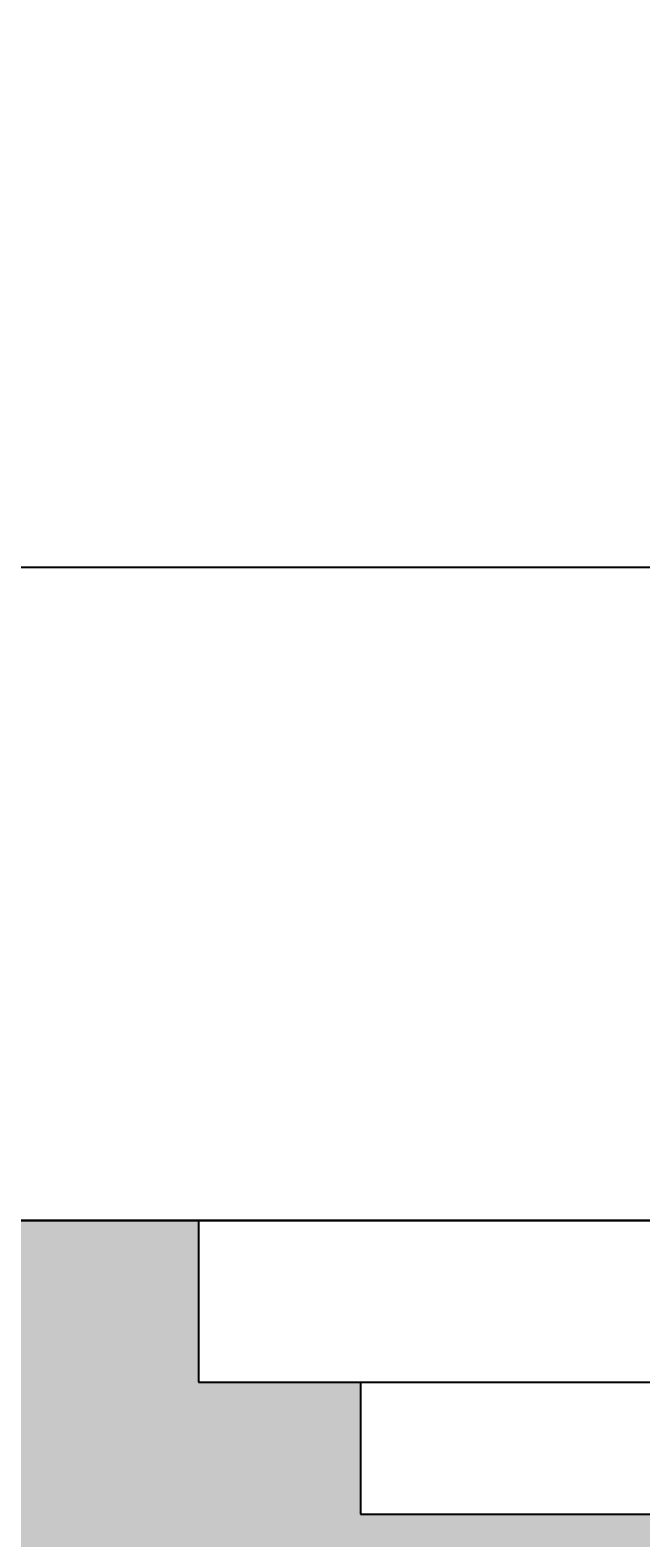
# Model space of a CAD drawing. Units: inches. Extents: x 2549 to 3108, y 1683 to 2362.
# Tile 5 of 30: x 2970 to 3018, y 1861 to 1979. Entities that reach past the tile are written whole.
import ezdxf

# ---------------------------------------------------------------- set-up
doc = ezdxf.new("R2010")
doc.units = ezdxf.units.IN
for name, color, linetype, lineweight in [('A-ANNO-DIMS', 2, 'Continuous', 18), ('A-FLOR', 7, 'Continuous', 25), ('A-FLOR-STRS', 7, 'Continuous', 25)]:
    doc.layers.add(name, color=color, linetype=linetype, lineweight=lineweight)
doc.layers.add('C-PKNG-VEHI-PATT', color=251, linetype='Continuous', lineweight=13, true_color=0x636466)
doc.layers.add('C-PVMT-PATT', color=9, linetype='Continuous', lineweight=13, true_color=0xc7c8ca)
doc.styles.get("Standard").update_dxf_attribs({"font": 'arial.ttf'})
doc.dimstyles.get("Standard").update_dxf_attribs({"dimtxt": 0.18, "dimasz": 0.18, "dimexe": 0.18, "dimexo": 0.0625, "dimgap": 0.09, "dimtad": 0, "dimtih": 1, "dimtoh": 1, "dimdec": 4, "dimzin": 0, "dimdsep": 46, "dimtxsty": 'Standard', "dimcen": 0.09, "dimadec": 0, "dimazin": 0, "dimtfac": 1, "dimtdec": 4, "dimtofl": 0, "dimtmove": 0, "dimatfit": 3, "dimfxl": 1, "dimtolj": 1, "dimtzin": 0, "dimarcsym": 0})

# ---------------------------------------------------------------- blocks, each defined once
blk = doc.blocks.new('*D46')
at = {"layer": 'A-ANNO-DIMS', "color": 0, "lineweight": -2, "transparency": 16777216}
for p, q in [((2812.642666, 2140.461244), (2812.642666, 1683.443744)), ((3034.642666, 2134.461244), (3034.642666, 1683.443744)), ((2812.822666, 1683.623744), (2923.35320488131, 1683.623744)), ((3034.462666, 1683.623744), (2923.932127118691, 1683.623744))]:
    blk.add_line(p, q, dxfattribs=at)
at = {"layer": 'A-ANNO-DIMS', "color": 0, "transparency": 16777216}
for points in [[(2812.822666, 1683.653744), (2812.822666, 1683.593744), (2812.642666, 1683.623744)], [(3034.462666, 1683.653744), (3034.462666, 1683.593744), (3034.642666, 1683.623744)]]:
    blk.add_solid(points, dxfattribs=at)
at = {"layer": 'Defpoints', "color": 0, "transparency": 16777216}
for p in [(2812.642666, 2140.523744), (3034.642666, 2134.523744), (3034.642666, 1683.623744)]:
    blk.add_point(p, dxfattribs=at)
at = {"layer": 'A-ANNO-DIMS', "color": 0, "transparency": 16777216, "insert": (2923.642666000001, 1683.623744), "char_height": 0.18, "attachment_point": 5}
blk.add_mtext('\\A1;222', dxfattribs=at)
blk = doc.blocks.new('*D56')
at = {"layer": 'A-ANNO-DIMS', "color": 0, "lineweight": -2, "transparency": 16777216}
for p, q in [((3043.580166000001, 1936.523744000001), (2549.424763000002, 1936.523744000001)), ((2549.604763000002, 1936.343744000001), (2549.604763000002, 1911.205647137791)), ((2549.604763000002, 1885.703744000001), (2549.604763000002, 1910.841840862211)), ((3043.580166000001, 1885.523744000001), (2549.424763000002, 1885.523744000001))]:
    blk.add_line(p, q, dxfattribs=at)
at = {"layer": 'A-ANNO-DIMS', "color": 0, "transparency": 16777216}
for points in [[(2549.574763000002, 1936.343744000001), (2549.634763000002, 1936.343744000001), (2549.604763000002, 1936.523744000001)], [(2549.574763000002, 1885.703744000001), (2549.634763000002, 1885.703744000001), (2549.604763000002, 1885.523744000001)]]:
    blk.add_solid(points, dxfattribs=at)
at = {"layer": 'Defpoints', "color": 0, "transparency": 16777216}
for p in [(2549.604763000002, 1936.523744000001), (3043.642666000001, 1936.523744000001), (3043.642666000001, 1885.523744000001)]:
    blk.add_point(p, dxfattribs=at)
at = {"layer": 'A-ANNO-DIMS', "color": 0, "transparency": 16777216, "insert": (2549.604763000002, 1911.023743999999), "char_height": 0.18, "attachment_point": 5}
blk.add_mtext('\\A1;51', dxfattribs=at)
blk = doc.blocks.new('*D57')
at = {"layer": 'A-ANNO-DIMS', "color": 0, "lineweight": -2, "transparency": 16777216}
for p, q in [((2965.93514, 1936.586244), (2965.93514, 2362.322518)), ((2966.11514, 2362.142518), (2999.912081717599, 2362.142518)), ((3034.462666, 2362.142518), (3000.665724282401, 2362.142518)), ((3034.642666, 1936.586244), (3034.642666, 2362.322518))]:
    blk.add_line(p, q, dxfattribs=at)
at = {"layer": 'A-ANNO-DIMS', "color": 0, "transparency": 16777216}
for points in [[(2966.11514, 2362.172518), (2966.11514, 2362.112518), (2965.93514, 2362.142518)], [(3034.462666, 2362.172518), (3034.462666, 2362.112518), (3034.642666, 2362.142518)]]:
    blk.add_solid(points, dxfattribs=at)
at = {"layer": 'Defpoints', "color": 0, "transparency": 16777216}
for p in [(3034.642666, 2362.142518), (2965.93514, 1936.523744), (3034.642666, 1936.523744)]:
    blk.add_point(p, dxfattribs=at)
at = {"layer": 'A-ANNO-DIMS', "color": 0, "transparency": 16777216, "insert": (3000.288903, 2362.142518), "char_height": 0.18, "attachment_point": 5}
blk.add_mtext('\\A1;68.71', dxfattribs=at)

msp = doc.modelspace()

# ---------------------------------------------------------------- hatches: boundary and pattern name
at = {"layer": 'C-PKNG-VEHI-PATT'}
h = msp.add_hatch(color=256, dxfattribs=at)
h.dxf.hatch_style = 1
edge = h.paths.add_edge_path()
edge.add_ellipse((2935.725796552836, 1791.96404850691), major_axis=(-50.6600031146233, 6.78e-13), ratio=0.8423038695439883, start_angle=248.1650462032912, end_angle=265.7225790369452)
edge.add_line((2938.911028887629, 1834.550737322417), (2925.865275339109, 1834.550737322417))
edge.add_ellipse((2929.050507673901, 1791.964048506909), major_axis=(50.66000311462998, 7.2698e-12), ratio=0.8423038695438956, start_angle=94.27742096304536, end_angle=111.8349537966996)
edge.add_line((2912.850791291541, 1832.394679033669), (2914.204376096751, 1822.249450253823))
edge.add_ellipse((2930.653832861207, 1783.102276333115), major_axis=(-49.30143828149606, 1.1087e-12), ratio=0.8423038695440098, start_angle=-85.12993040286318, end_angle=-67.20808512241217, ccw=False)
edge.add_line((2927.124659327709, 1824.522535937876), (2937.65164489903, 1824.522535937876))
edge.add_ellipse((2934.122471365533, 1783.102276333124), major_axis=(49.30143828148681, 7.803e-13), ratio=0.8423038695439693, start_angle=67.20808512240922, end_angle=85.12993040286312, ccw=False)
edge.add_line((2950.571928129987, 1822.249450253823), (2951.925512935197, 1832.394679033669))
edge = h.paths.add_edge_path()
edge.add_ellipse((2903.479330909537, 1857.335124490177), major_axis=(-34.79790434319148, 3.2087e-12), ratio=0.8423038695440206, start_angle=180.0000000000052, end_angle=209.4385695979841)
edge.add_ellipse((2961.296973317201, 1857.335124490177), major_axis=(34.79790434319149, 1.2616e-12), ratio=0.8423038695439669, start_angle=150.5614304020187, end_angle=179.9999999999979)
edge.add_line((2926.49906897401, 1857.335124490177), (2926.49906897401, 1843.76085484809))
edge.add_ellipse((2924.125124210826, 1844.314306179491), major_axis=(-0.2209272451118966, 3.927824345135514), ratio=0.6038335755719296, start_angle=89.00201427502537, end_angle=253.65740804569998, ccw=False)
edge.add_line((2921.751179447642, 1844.222223668088), (2921.751179447642, 1853.39746861696))
edge.add_line((2921.751179447642, 1853.39746861696), (2925.26903797625, 1855.848425453852))
edge.add_ellipse((2925.478177919096, 1855.493055533625), major_axis=(0.4583993962922678, 2.303e-12), ratio=0.8423038695418179, start_angle=89.9999999997122, end_angle=134.4802108822853, ccw=False)
edge.add_line((2925.478177919095, 1855.879167118917), (2926.49906897401, 1855.879167118917))
edge.add_line((2926.49906897401, 1855.879167118917), (2926.49906897401, 1857.335124490177))
edge.add_ellipse((2961.296973317201, 1857.335124490177), major_axis=(34.79790434319149, 1.2616e-12), ratio=0.8423038695439669, start_angle=150.5614304020187, end_angle=179.999999999998, ccw=False)
edge.add_line((2932.388152113369, 1873.650056952746), (2932.388152113369, 1875.780055063896))
edge.add_ellipse((2932.388152113369, 1875.393943478604), major_axis=(0.4583993962904624, 1e-16), ratio=0.8423038695446395, start_angle=89.99999999999999, end_angle=127.9331304598429)
edge.add_line((2932.136581844764, 1875.716714504374), (2928.591534983032, 1873.756406364807))
edge.add_ellipse((2899.927094610101, 2002.469218934773), major_axis=(155.4756451483881, 9.82606e-11), ratio=0.842303869543439, start_angle=-80.74343399283458, end_angle=-77.44506735589891, ccw=False)
edge.add_ellipse((2949.440169726089, 1715.215149574257), major_axis=(-189.1421864819335, 9.35831e-11), ratio=0.8423038695443681, start_angle=-79.79046100282835, end_angle=-77.55537270652765)
edge.add_ellipse((3300.361430890526, 1852.564199885104), major_axis=(-386.1662101011402, 3.282e-12), ratio=0.8423038695438535, start_angle=-2.863714607837213, end_angle=2.198540565955553)
edge.add_ellipse((2929.050507673902, 1792.515918881865), major_axis=(-55.61920468847034, 9.624e-12), ratio=0.842303869544118, start_angle=-85.91758930883981, end_angle=-72.28004677724027, ccw=False)
edge.add_line((2925.712863234435, 1839.27976237288), (2939.063440992303, 1839.27976237288))
edge.add_ellipse((2935.725796552836, 1792.515918881865), major_axis=(55.61920468846977, 1.19088e-11), ratio=0.8423038695441256, start_angle=72.28004677723749, end_angle=85.91758930883759, ccw=False)
edge.add_ellipse((2564.414873336211, 1852.564199885105), major_axis=(-386.166210101141, 7.3121e-12), ratio=0.8423038695442235, start_angle=177.8014594340458, end_angle=182.8637146078386)
edge.add_ellipse((2915.336134500645, 1715.215149574254), major_axis=(189.1421864814668, 5.425418e-10), ratio=0.8423038695464061, start_angle=77.5553727063904, end_angle=79.79046100269107)
edge.add_ellipse((2964.849209616638, 2002.469218934773), major_axis=(-155.4756451483861, 9.70869e-11), ratio=0.8423038695434499, start_angle=77.44506735589852, end_angle=80.74343399283418, ccw=False)
edge.add_line((2936.184769243706, 1873.756406364807), (2932.639722381973, 1875.716714504375))
edge.add_ellipse((2932.388152113369, 1875.393943478604), major_axis=(0.4583993962904624, 1e-16), ratio=0.8423038695446395, start_angle=52.06686954015704, end_angle=89.99999999999999)
edge.add_line((2932.388152113369, 1875.780055063896), (2932.388152113369, 1873.650056952746))
edge.add_ellipse((2903.479330909537, 1857.335124490177), major_axis=(-34.79790434319148, 3.2087e-12), ratio=0.8423038695440206, start_angle=180.0000000000053, end_angle=209.4385695979841, ccw=False)
edge.add_line((2938.277235252728, 1857.335124490177), (2938.277235252728, 1855.879167118917))
edge.add_line((2938.277235252728, 1855.879167118917), (2939.405880844674, 1855.879167118917))
edge.add_ellipse((2939.298126307642, 1855.493055533625), major_axis=(-0.4583993962922676, 2.3028e-12), ratio=0.8423038695418185, start_angle=225.5197891177147, end_angle=270.00000000028786, ccw=False)
edge.add_line((2939.590297193029, 1855.790576266728), (2943.025124779096, 1853.39746861696))
edge.add_line((2943.025124779096, 1853.39746861696), (2943.025124779096, 1844.222223668088))
edge.add_ellipse((2940.651180015912, 1844.314306179491), major_axis=(0.2209272451118966, 3.927824345135514), ratio=0.6038335755719296, start_angle=106.3425919543001, end_angle=270.9979857249746, ccw=False)
edge.add_line((2938.277235252728, 1843.76085484809), (2938.277235252728, 1857.335124490177))
edge = h.paths.add_edge_path()
edge.add_ellipse((2932.388152113369, 1865.19731394932), major_axis=(91.08099646002908, 7.134e-13), ratio=0.8423038695439837, start_angle=256.4018653097688, end_angle=283.5981346902299, ccw=False)
edge.add_line((2914.204376096751, 1790.023884530285), (2914.204376096751, 1778.36217788565))
edge.add_ellipse((2932.388152113369, 1853.535607304685), major_axis=(91.08099646002908, 7.134e-13), ratio=0.8423038695439837, start_angle=256.4018653097688, end_angle=283.5981346902299)
edge.add_line((2950.571928129987, 1778.36217788565), (2950.571928129987, 1790.023884530285))
edge = h.paths.add_edge_path()
edge.add_ellipse((2948.738330544823, 1772.31452600415), major_axis=(1.833597585163715, 1.1861e-12), ratio=0.8423038695440299, start_angle=-3.70558e-11, end_angle=89.99999999996297)
edge.add_line((2948.738330544824, 1773.85897234532), (2916.037973681915, 1773.858972345321))
edge.add_ellipse((2916.037973681915, 1772.314526004151), major_axis=(1.833597585163716, 6.788e-13), ratio=0.84230386954403, start_angle=89.9999999999788, end_angle=179.9999999999787)
edge.add_line((2914.204376096751, 1772.314526004151), (2914.204376096751, 1760.255799913309))
edge.add_line((2914.204376096751, 1760.255799913309), (2950.571928129987, 1760.255799913308))
edge.add_line((2950.571928129987, 1760.255799913308), (2950.571928129987, 1772.31452600415))
h.paths.add_polyline_path([(2748.849609196547, 2101.638310911291), (2798.147998217048, 2101.638310911291), (2798.147998217048, 2111.424826549233), (2748.849609196547, 2111.424826549233)], flags=9)
h.paths.add_polyline_path([(2685.208067619545, 2101.488974631509), (2719.325307162104, 2101.488974631509), (2719.325307162104, 2111.281945754699), (2685.208067619545, 2111.281945754699)], flags=9)
h.paths.add_polyline_path([(2814.685179139321, 1907.132804880864), (2847.838399551318, 1907.132804880864), (2847.838399551318, 1916.925776004054), (2814.685179139321, 1916.925776004054)], flags=9)
h.paths.add_polyline_path([(2814.390575309562, 1835.586397562281), (2848.017197973174, 1835.586397562281), (2848.017197973174, 1845.379368685471), (2814.390575309562, 1845.379368685471)], flags=9)
h.paths.add_polyline_path([(2800.524456569608, 1759.167447237475), (2853.743476964851, 1759.167447237475), (2853.743476964851, 1768.953962875417), (2800.524456569608, 1768.953962875417)], flags=9)
h.paths.add_polyline_path([(2972.461062245805, 1807.33049128039), (3015.394342810494, 1807.33049128039), (3015.394342810494, 1817.117006918332), (2972.461062245805, 1817.117006918332)], flags=9)
h.paths.add_polyline_path([(2902.332650472062, 1888.673085326325), (2937.913133337796, 1888.673085326325), (2937.913133337796, 1898.466056449515), (2902.332650472062, 1898.466056449515)], flags=9)
h.paths.add_polyline_path([(2712.17793111998, 1878.903902566108), (2754.125674269943, 1878.903902566108), (2754.125674269943, 1888.69041820405), (2712.17793111998, 1888.69041820405)], flags=9)
h.paths.add_polyline_path([(2614.005606808349, 2012.811964980989), (2650.025062671036, 2012.811964980989), (2650.025062671036, 2022.437093487698), (2614.005606808349, 2022.437093487698)], flags=9)
h.paths.add_polyline_path([(2713.312922761346, 2003.164487508756), (2747.423706818656, 2003.164487508756), (2747.423706818656, 2012.951003146698), (2713.312922761346, 2012.951003146698)], flags=9)
h.paths.add_polyline_path([(2950.137937233872, 2001.693439459313), (2982.299164745893, 2001.693439459313), (2982.299164745893, 2011.479955097255), (2950.137937233872, 2011.479955097255)], flags=9)
h.paths.add_polyline_path([(2940.863994744806, 2238.553674899427), (2997.506574150595, 2238.553674899427), (2997.506574150595, 2248.346646022617), (2940.863994744806, 2248.346646022617)], flags=9)
h.paths.add_polyline_path([(2821.545730132573, 2202.834824551463), (2855.662969675132, 2202.834824551463), (2855.662969675132, 2212.627795674654), (2821.545730132573, 2212.627795674654)], flags=9)
h.paths.add_polyline_path([(2661.802564922812, 2238.624912952816), (2718.445144328601, 2238.624912952816), (2718.445144328601, 2248.417884076006), (2661.802564922812, 2248.417884076006)], flags=9)
at = {"layer": 'C-PVMT-PATT'}
h = msp.add_hatch(color=256, dxfattribs=at)
h.dxf.hatch_style = 1
h.paths.add_polyline_path([(3067.642666391656, 2305.523744486262), (2605.642666391656, 2305.523744486262), (2605.642666391656, 2074.523744486262), (2629.642666391656, 2074.523744486262), (2629.642666391656, 2281.523744486262), (3043.642666391656, 2281.523744486262), (3043.642666391656, 1885.523744486263), (3043.642666391656, 1872.874514030248), (3031.167181590035, 1872.874514030248), (3031.167181590035, 1862.573058982011), (2995.805391311171, 1862.573058982011), (2995.805391311171, 1872.874514030248), (2983.175155144805, 1872.874514030248), (2983.175155144805, 1885.523744486262), (2881.642666391656, 1885.523744486263), (2881.642666391656, 1795.523744486262), (2751.09773888662, 1795.523744486262), (2751.09773888662, 1761.523744486262), (2786.157685455576, 1761.523744486262), (2786.157685455577, 1723.523744486262), (2881.839988255281, 1723.523744486262), (2881.839988255281, 1714.523744486262), (3067.642666391656, 1714.523744486262), (3067.642666391656, 1723.523744486262)])
edge = h.paths.add_edge_path(flags=16)
edge.add_ellipse((2949.440169726093, 1710.96831784248), major_axis=(-194.1013880556022, 3.100242e-10), ratio=0.8423038695451509, start_angle=-77.87403444762441, end_angle=-76.21947101041059, ccw=False)
edge.add_ellipse((2949.440169726089, 1715.215149574257), major_axis=(-189.1421864819335, 9.35831e-11), ratio=0.8423038695443681, start_angle=-79.7904610028283, end_angle=-77.55537270652758, ccw=False)
edge.add_ellipse((2899.927094610101, 2002.469218934773), major_axis=(155.4756451483881, 9.82606e-11), ratio=0.842303869543439, start_angle=-80.74343399283462, end_angle=-77.44506735589897)
edge.add_line((2928.591534983032, 1873.756406364807), (2932.388152113369, 1875.855825569603))
edge.add_line((2932.388152113369, 1875.855825569603), (2936.184769243706, 1873.756406364807))
edge.add_ellipse((2964.849209616638, 2002.469218934773), major_axis=(-155.4756451483861, 9.70869e-11), ratio=0.8423038695434499, start_angle=77.4450673558985, end_angle=80.74343399283416)
edge.add_ellipse((2915.336134500645, 1715.215149574254), major_axis=(189.1421864814668, 5.425418e-10), ratio=0.8423038695464061, start_angle=77.55537270639041, end_angle=79.79046100269102, ccw=False)
edge.add_ellipse((2915.336134500645, 1710.96831784248), major_axis=(-194.1013880561466, 2.794238e-10), ratio=0.8423038695428703, start_angle=256.2194710105847, end_angle=257.8740344477983, ccw=False)
edge.add_ellipse((2628.287132012546, 1850.261185811051), major_axis=(-327.2531525161749, 1.24457e-11), ratio=0.8423038695440036, start_angle=182.1799503136474, end_angle=183.6504275857012, ccw=False)
edge.add_ellipse((2955.563661936079, 1861.933375066942), major_axis=(-0.9167987925820851, 6.203e-13), ratio=0.8423038695438211, start_angle=180.0000000000388, end_angle=270.00000000003877, ccw=False)
edge.add_line((2956.480460728661, 1862.385732927092), (2956.480460728661, 1846.486613953928))
edge.add_ellipse((2955.563661936079, 1846.938971814078), major_axis=(-0.9167987925816303, 6.983e-13), ratio=0.8423038695442389, start_angle=90.0000000000436, end_angle=180.0000000000437, ccw=False)
edge.add_ellipse((-3607.060581297885, 1835.831972437108), major_axis=(-6562.624243233964, 2.000376e-10), ratio=0.8423038695434055, start_angle=179.6161332212093, end_angle=180.0902290885961, ccw=False)
edge.add_ellipse((2955.563661936079, 1791.092611498023), major_axis=(0.9167987925816303, 1.8053e-12), ratio=0.8423038695442389, start_angle=-1.127773430198431e-10, end_angle=89.99999999988711, ccw=False)
edge.add_line((2956.480460728661, 1791.544969358173), (2956.480460728661, 1775.645850385008))
edge.add_ellipse((2955.563661936079, 1776.098208245159), major_axis=(0.9167987925816303, 5.91e-14), ratio=0.8423038695442391, start_angle=269.9999999999963, end_angle=359.9999999999963, ccw=False)
edge.add_ellipse((-3607.060581297885, 1835.831972437108), major_axis=(-6562.624243233964, 2.000376e-10), ratio=0.8423038695434055, start_angle=179.3813568036826, end_angle=179.4717285281838, ccw=False)
edge.add_ellipse((2954.590723441648, 1763.876816393945), major_axis=(-1.375198188872997, 3.586e-13), ratio=0.8423038695436877, start_angle=179.3717627838213, end_angle=248.4647566010281, ccw=False)
edge.add_ellipse((-3607.518980694323, 1835.831972435604), major_axis=(-6564.040927375597, 4.0829067806e-06), ratio=0.8423038626957529, start_angle=179.3534459385899, end_angle=179.371762819423, ccw=False)
edge.add_ellipse((2952.682914207262, 1761.800246254478), major_axis=(3.250281735962, 3.921e-13), ratio=0.8423038695438826, start_angle=-89.99999999994031, end_angle=-0.6465540970884831, ccw=False)
edge.add_line((2952.682914207266, 1759.06252137117), (2912.093390019471, 1759.062521371171))
edge.add_ellipse((2912.093390019478, 1761.800246254481), major_axis=(3.250281735963338, 1.2841e-12), ratio=0.8423038695440954, start_angle=180.6465540970387, end_angle=269.99999999984414, ccw=False)
edge.add_ellipse((9472.295284948175, 1835.831972439052), major_axis=(-6564.040927413921, 8.323842912e-07), ratio=0.8423038709559154, start_angle=0.6282372235086768, end_angle=0.646554104341817, ccw=False)
edge.add_ellipse((2910.185580785089, 1763.876816393947), major_axis=(1.375198188873441, 9.687e-13), ratio=0.8423038695438604, start_angle=111.53524350397811, end_angle=180.6282372161342, ccw=False)
edge.add_ellipse((9471.836885542962, 1835.831972437208), major_axis=(-6562.624243252301, 3.836442e-10), ratio=0.8423038695462286, start_angle=0.5282714718206876, end_angle=0.6465540970643247, ccw=False)
edge.add_ellipse((2909.212642290659, 1776.098208245159), major_axis=(-0.9167987925820851, 6.203e-13), ratio=0.8423038695438211, start_angle=3.8824055081931874e-11, end_angle=90.00000000003882, ccw=False)
edge.add_line((2908.295843498077, 1775.645850385009), (2908.295843498077, 1791.544969358173))
edge.add_ellipse((2909.212642290659, 1791.092611498023), major_axis=(-0.9167987925820851, 4.868e-13), ratio=0.8423038695438213, start_angle=-89.99999999996948, end_angle=3.041122909053229e-11, ccw=False)
edge.add_ellipse((9471.836885542962, 1835.831972437208), major_axis=(-6562.624243252301, 3.836442e-10), ratio=0.8423038695462286, start_angle=-0.09022908858980827, end_angle=0.38386677879560693, ccw=False)
edge.add_ellipse((2909.212642290658, 1846.938971814078), major_axis=(-0.9167987925816306, 1.1661e-12), ratio=0.8423038695442389, start_angle=7.287326297955588e-11, end_angle=90.00000000007287, ccw=False)
edge.add_line((2908.295843498077, 1846.486613953928), (2908.295843498077, 1862.385732927092))
edge.add_ellipse((2909.212642290658, 1861.933375066942), major_axis=(0.9167987925816303, 1.1659e-12), ratio=0.8423038695442391, start_angle=89.99999999992713, end_angle=179.9999999999272, ccw=False)
edge.add_ellipse((3236.489172214191, 1850.261185811051), major_axis=(327.2531525161745, 3.33005e-11), ratio=0.8423038695444386, start_angle=176.3495724142951, end_angle=177.820049686349, ccw=False)
edge = h.paths.add_edge_path(flags=0)
edge.add_ellipse((2903.479330909537, 1857.335124490177), major_axis=(-34.79790434319148, 3.2087e-12), ratio=0.8423038695440206, start_angle=180.0000000000053, end_angle=209.4385695979841, ccw=False)
edge.add_line((2938.277235252728, 1857.335124490177), (2938.277235252728, 1855.879167118917))
edge.add_line((2938.277235252728, 1855.879167118917), (2939.463142736354, 1855.879167118917))
edge.add_line((2939.463142736354, 1855.879167118917), (2943.025124779096, 1853.39746861696))
edge.add_line((2943.025124779096, 1853.39746861696), (2943.025124779096, 1844.222223668088))
edge.add_ellipse((2940.651180015912, 1844.314306179491), major_axis=(0.2209272451118966, 3.927824345135514), ratio=0.6038335755719296, start_angle=106.3425919543001, end_angle=270.9979857249746, ccw=False)
edge.add_line((2938.277235252728, 1843.76085484809), (2938.277235252728, 1857.335124490177))
edge.add_ellipse((2903.479330909537, 1857.335124490177), major_axis=(-34.79790434319148, 3.2087e-12), ratio=0.8423038695440206, start_angle=180.0000000000052, end_angle=209.4385695979841)
edge.add_ellipse((2961.296973317201, 1857.335124490177), major_axis=(34.79790434319149, 1.2616e-12), ratio=0.8423038695439669, start_angle=150.5614304020187, end_angle=179.9999999999979)
edge.add_line((2926.49906897401, 1857.335124490177), (2926.49906897401, 1843.76085484809))
edge.add_ellipse((2924.125124210826, 1844.314306179491), major_axis=(-0.2209272451118966, 3.927824345135514), ratio=0.6038335755719296, start_angle=89.00201427502537, end_angle=253.65740804569998, ccw=False)
edge.add_line((2921.751179447642, 1844.222223668088), (2921.751179447642, 1853.39746861696))
edge.add_line((2921.751179447642, 1853.39746861696), (2925.313161490385, 1855.879167118917))
edge.add_line((2925.313161490385, 1855.879167118917), (2926.49906897401, 1855.879167118917))
edge.add_line((2926.49906897401, 1855.879167118917), (2926.49906897401, 1857.335124490177))
edge.add_ellipse((2961.296973317201, 1857.335124490177), major_axis=(34.79790434319149, 1.2616e-12), ratio=0.8423038695439669, start_angle=150.5614304020187, end_angle=179.999999999998, ccw=False)
edge = h.paths.add_edge_path(flags=0)
edge.add_ellipse((2929.050507673901, 1791.964048506909), major_axis=(50.66000311462998, 7.2698e-12), ratio=0.8423038695438956, start_angle=94.2774209630453, end_angle=111.8349537966997, ccw=False)
edge.add_line((2925.865275339109, 1834.550737322417), (2938.911028887629, 1834.550737322417))
edge.add_ellipse((2935.725796552836, 1791.96404850691), major_axis=(-50.6600031146233, 6.78e-13), ratio=0.8423038695439883, start_angle=248.16504620329118, end_angle=265.72257903694526, ccw=False)
edge.add_line((2951.925512935197, 1832.394679033669), (2950.571928129987, 1822.249450253823))
edge.add_ellipse((2934.122471365533, 1783.102276333124), major_axis=(49.30143828148681, 7.803e-13), ratio=0.8423038695439693, start_angle=67.20808512240917, end_angle=85.12993040286312)
edge.add_line((2937.651644899029, 1824.522535937876), (2927.12465932771, 1824.522535937876))
edge.add_ellipse((2930.653832861207, 1783.102276333115), major_axis=(-49.30143828149606, 1.1087e-12), ratio=0.8423038695440098, start_angle=-85.12993040286322, end_angle=-67.20808512241221)
edge.add_line((2914.204376096751, 1822.249450253823), (2912.850791291541, 1832.394679033669))
edge = h.paths.add_edge_path(flags=0)
edge.add_line((2910.133794844343, 1829.46512489105), (2912.643202843121, 1821.271117801794))
edge.add_ellipse((5203.77865552976, 1816.436683891122), major_axis=(-2291.142641748503, 9.8835e-11), ratio=0.8423038695495838, start_angle=-0.1208973690305054, end_angle=0.3640763488925343)
edge.add_line((2912.701209242743, 1801.878223466977), (2910.33046059899, 1792.569831244782))
edge.add_ellipse((9471.836885542954, 1835.831972437156), major_axis=(-6561.70744445971, 7.61654e-11), ratio=0.8423038695443023, start_angle=0.055594313499796044, end_angle=0.37776419391019544, ccw=False)
edge = h.paths.add_edge_path(flags=0)
edge.add_ellipse((-3607.060581316224, 1835.831972437187), major_axis=(6561.707444459722, 1.43187e-10), ratio=0.8423038695443235, start_angle=-0.37776419391110494, end_angle=-0.05559431350059185, ccw=False)
edge.add_line((2954.445843627751, 1792.569831244769), (2952.075094983995, 1801.878223466976))
edge.add_ellipse((660.9976486969767, 1816.436683891133), major_axis=(2291.142641748505, 5.276994e-10), ratio=0.842303869552366, start_angle=-0.3640763489035208, end_angle=0.1208973690194708)
edge.add_line((2952.133101383619, 1821.2711178018), (2954.642509382395, 1829.46512489105))
edge = h.paths.add_edge_path(flags=0)
edge.add_ellipse((2932.388152113369, 1865.19731394932), major_axis=(91.08099646002908, 7.134e-13), ratio=0.8423038695439837, start_angle=256.4018653097688, end_angle=283.5981346902299)
edge.add_line((2950.571928129987, 1790.023884530285), (2950.571928129987, 1778.362177885651))
edge.add_ellipse((2932.388152113369, 1853.535607304685), major_axis=(91.08099646002908, 7.134e-13), ratio=0.8423038695439837, start_angle=256.4018653097688, end_angle=283.5981346902299, ccw=False)
edge.add_line((2914.204376096751, 1778.362177885651), (2914.204376096751, 1790.023884530285))
edge = h.paths.add_edge_path(flags=0)
edge.add_line((2916.037973681915, 1773.858972345321), (2948.738330544823, 1773.85897234532))
edge.add_ellipse((2948.738330544823, 1772.31452600415), major_axis=(1.833597585163715, 1.1861e-12), ratio=0.8423038695440299, start_angle=-3.7118752516107634e-11, end_angle=89.999999999963, ccw=False)
edge.add_line((2950.571928129987, 1772.31452600415), (2950.571928129987, 1760.255799913308))
edge.add_line((2950.571928129987, 1760.255799913308), (2914.204376096751, 1760.255799913309))
edge.add_line((2914.204376096751, 1760.255799913309), (2914.204376096751, 1772.314526004151))
edge.add_ellipse((2916.037973681915, 1772.314526004151), major_axis=(1.833597585163716, 6.788e-13), ratio=0.84230386954403, start_angle=89.9999999999788, end_angle=179.9999999999788, ccw=False)
h.paths.add_polyline_path([(2629.642666391656, 1978.523744486262), (2605.642666391656, 1978.523744486262), (2605.642666391656, 1723.523744486262), (2629.642666391656, 1723.523744486262), (2629.642666391656, 1795.523744486262)], flags=17)
h.paths.add_polyline_path([(2800.524456569608, 1759.167447237475), (2853.743476964851, 1759.167447237475), (2853.743476964851, 1768.953962875417), (2800.524456569608, 1768.953962875417)], flags=24)
h.paths.add_polyline_path([(2972.461062245805, 1807.33049128039), (3015.394342810494, 1807.33049128039), (3015.394342810494, 1817.117006918332), (2972.461062245805, 1817.117006918332)], flags=24)

# ---------------------------------------------------------------- linework, layer by layer
at = {"layer": 'A-FLOR'}
msp.add_line((2881.642666391656, 1885.523744486263), (3043.642666391656, 1885.523744486262), dxfattribs=at)
at = {"layer": 'A-FLOR-STRS'}
for p, q in [((2983.175155144805, 1885.523744486262), (2983.175155144805, 1872.874514030248)), ((2983.175155144805, 1872.874514030248), (3043.642666391656, 1872.874514030248)), ((2995.805391311171, 1872.874514030248), (2995.805391311171, 1862.573058982011)), ((2995.805391311171, 1862.573058982011), (3031.167181590035, 1862.573058982011))]:
    msp.add_line(p, q, dxfattribs=at)

# ---------------------------------------------------------------- dimensions: what is measured, and where the dimension line sits
at = {"layer": 'A-ANNO-DIMS'}
for base, p1, p2, override, picture, middle in [((3034.642666, 2362.142518), (2965.93514, 1936.523744), (3034.642666, 1936.523744), {"dimdec": 2, "dimlfac": 1, "dimrnd": 0, "dimzin": 0, "dimdsep": 46, "dimlunit": 2}, '*D57', (3000.288903, 2362.142518)), ((3034.642666, 1683.623744), (2812.642666, 2140.523744), (3034.642666, 2134.523744), {"dimdec": 0, "dimlfac": 1, "dimrnd": 0, "dimzin": 0, "dimdsep": 46, "dimlunit": 2}, '*D46', (2923.642666000001, 1683.623744))]:
    dim = msp.add_linear_dim(base=base, p1=p1, p2=p2, dimstyle='Standard', override=override, dxfattribs=at)
    dim.commit()
    dim.dimension.update_dxf_attribs({"geometry": picture, "text_midpoint": middle})
dim = msp.add_linear_dim(base=(2549.604763000002, 1936.523744000001), p1=(3043.642666, 1885.523744), p2=(3043.642666, 1936.523744), angle=90, dimstyle='Standard', override={"dimdec": 0, "dimlfac": 1, "dimrnd": 0, "dimzin": 0, "dimdsep": 46, "dimlunit": 2}, dxfattribs=at)
dim.commit()
dim.dimension.update_dxf_attribs({"geometry": '*D56', "text_midpoint": (2549.604763000002, 1911.023743999999)})

doc.saveas('drawing.dxf')
